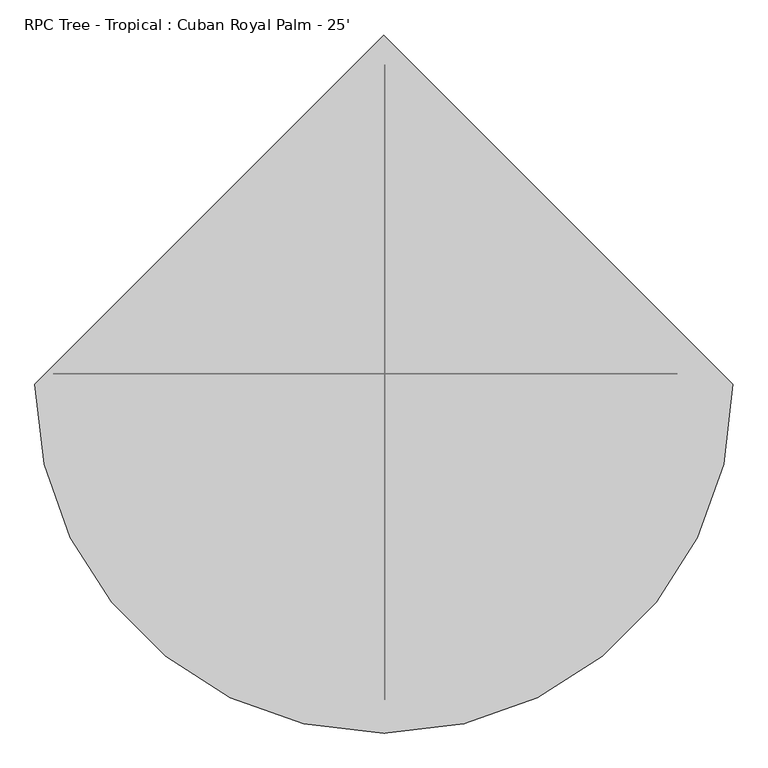
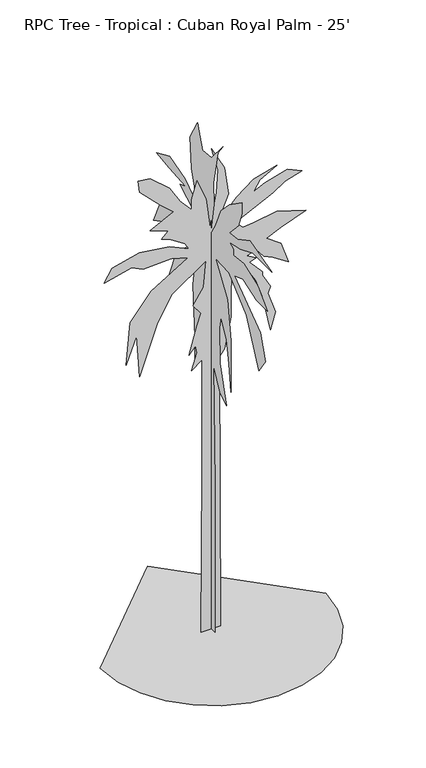
"""IFC4 building model written with IfcOpenShell, lengths in millimetres: geographic element geometry, RPC Tree - Tropical : Cuban Royal Palm - 25'."""

from ifc_helpers import new_model, si_unit, origin, place, context, project, spatial, triangles, source, transform, mapped, element, save


def rpc_tree_tropical_cuban_royal_palm_25_0a7aa95b(model_context):
    return source(origin(), model_context, "Body", "Tessellation", [
        triangles([(-108.765227, -0.0349819, 0.0018874), (-300.0839361, -0.0349989, 0.0018958), (-261.8198836, -0.0358763, 4989.2966217), (-261.8193749, -0.0364853, 8394.7422455), (-567.9281977, -0.0364309, 8165.1771881), (-414.8755486, -0.0365265, 8662.6107788), (-453.138075, -0.0365659, 8892.1752548), (-644.4583374, -0.0365165, 8662.6107788), (-414.8750399, -0.036677, 9504.4163727), (-300.0834274, -0.0367436, 9848.7895386), (-529.6656713, -0.0367883, 10154.9103882), (-223.556358, -0.0368838, 10614.0393402), (-147.0287708, -0.0370308, 11417.5937805), (-1141.8863325, -0.0368642, 10728.8474487), (-1562.7842606, -0.0367158, 10001.8499634), (-2098.4799053, -0.0364255, 8509.550354), (-2175.0048855, -0.0366548, 9810.5372223), (-2481.1151253, -0.0364977, 9006.9833633), (-2366.327655, -0.0367286, 10269.667337), (-1754.1070301, -0.0368921, 11034.9682983), (-682.7208275, -0.0370553, 11685.4611511), (-1180.1488953, -0.037061, 11838.5215759), (-1983.6872028, -0.037019, 11800.2181), (-2328.060078, -0.0370313, 11953.2785248), (-3131.5983856, -0.0369619, 11761.9657837), (-2902.0182129, -0.0370404, 12144.5912659), (-2098.4799053, -0.0371098, 12335.9551666), (-1218.4113853, -0.0371277, 12221.1470581), (-644.4583374, -0.0371049, 11953.2785248), (-759.2509672, -0.0371341, 12144.5912659), (-1218.4113853, -0.0371687, 12450.7121155), (-1447.996645, -0.0371724, 12527.2679077), (-1256.6789623, -0.037215, 12718.5806488), (-1792.3695202, -0.0372257, 12909.8922272), (-1103.6238424, -0.0373174, 13254.2653931), (-1486.2591351, -0.0373623, 13598.638559), (-2098.4799053, -0.037445, 14210.8790955), (-2136.7423954, -0.0375049, 14555.2522614), (-1792.3695202, -0.0375131, 14516.9487854), (-1218.4113853, -0.0374493, 14019.5163574), (-912.3010729, -0.0373737, 13522.0827667), (-567.9281977, -0.0373203, 13139.4572845), (-567.9281977, -0.037375, 13445.5781342), (-414.8750399, -0.0374776, 13981.2640411), (-147.0287708, -0.037373, 13330.7700256), (-32.2376989, -0.0372138, 12412.4597992), (159.0810602, -0.0374, 13407.3258179), (197.3450945, -0.0375249, 14096.0709869), (6.0263474, -0.0376465, 14823.069635), (388.6638127, -0.0375332, 14096.0709869), (503.4554252, -0.0373877, 13254.2653931), (159.0810602, -0.0372221, 12412.4597992), (733.0381777, -0.0373635, 13062.952652), (1230.4661728, -0.0374537, 13445.5781342), (1919.2119232, -0.037518, 13636.8908752), (1421.7838554, -0.0374483, 13369.0735016), (1230.4661728, -0.0373853, 13062.952652), (1574.839048, -0.0374277, 13216.0130768), (2225.3223083, -0.0374903, 13407.3258179), (2646.2251053, -0.0374745, 13216.0130768), (2148.7971828, -0.0374254, 13062.952652), (1804.4243076, -0.0373693, 12833.3375977), (694.7756876, -0.037225, 12297.6516907), (924.3558603, -0.037194, 12068.0866333), (1230.4661728, -0.0372142, 12106.3389496), (1919.2119232, -0.0372649, 12221.1470581), (2761.0178078, -0.0372537, 11953.2785248), (2034.0046257, -0.0371741, 11685.4611511), (1613.1015381, -0.0371215, 11494.14841), (2034.0046257, -0.0370851, 11188.0287231), (2263.5847984, -0.0369789, 10537.5347076), (1804.4243076, -0.0370135, 10843.6555573), (1536.5765579, -0.0370223, 10958.4125061), (1230.4661728, -0.0370774, 11341.0891479), (1230.4661728, -0.0370568, 11226.2810394), (1039.1484901, -0.0370348, 11149.7764069), (1306.9912983, -0.0370191, 10996.7159821), (1115.673543, -0.0369971, 10920.1601898), (1498.3140678, -0.0369385, 10499.2823914), (1498.3140678, -0.036918, 10384.4742828), (1727.8942406, -0.0368528, 9963.5976471), (1651.3692604, -0.0368152, 9772.284906), (1880.9494331, -0.036709, 9121.7914719), (1727.8942406, -0.0366133, 8624.3584625), (1498.3140678, -0.0368017, 9733.9814301), (1306.9912983, -0.036896, 10307.9696503), (962.6184231, -0.0369835, 10881.9078735), (618.2455479, -0.0369959, 11034.9682983), (579.9830215, -0.0368573, 10269.667337), (579.9830215, -0.0367068, 9427.9117401), (388.6638127, -0.0365343, 8509.550354), (235.6086383, -0.0364934, 8318.2376129), (273.8721821, -0.0350103, 0.0018707), (-0.007416, 179.1973287, 0.0009899), (-0.0074167, 327.2669789, 0.0010164), (-0.007416, 327.2669789, 3653.5578049), (-0.007412, 290.2500887, 8576.860199), (-0.0074152, 438.3187397, 8354.762709), (-0.0074113, 808.4913483, 7577.3712067), (-0.0074142, 808.4913483, 8502.8449493), (-0.0074136, 919.5451075, 10057.5767944), (-0.0074165, 771.4734043, 11131.0821991), (-0.0074182, 1067.6117237, 10797.8850952), (-0.0074135, 1585.8575615, 9724.3802719), (-0.0074128, 2178.1342003, 8984.0725525), (-0.0074169, 2622.3390633, 8280.7474594), (-0.0074142, 2104.0983124, 9687.3976456), (-0.0074148, 1770.942049, 10501.7717743), (-0.0074148, 1030.5937798, 11242.130072), (-0.007418, 1363.7500431, 11168.0636627), (-0.0074146, 1807.959993, 11131.0821991), (-0.0074152, 2215.1521442, 11205.0974487), (-0.0074151, 2918.4826149, 10834.9177185), (-0.0074174, 2548.3084076, 11649.2924286), (-0.0074135, 2141.1162563, 11649.2924286), (-0.0074142, 1993.0446259, 12278.6016907), (-0.0074152, 1289.7192421, 12130.5200317), (-0.0074177, 845.5092922, 12352.6169403), (-0.0074181, 1585.8575615, 12759.8292938), (-0.0074118, 1289.7192421, 12870.8783295), (-0.0074163, 2104.0983124, 12944.8935791), (-0.0074128, 2770.4108391, 13018.9599884), (-0.0074146, 2104.0983124, 13315.0733093), (-0.0074149, 1326.7371861, 13092.975238), (-0.0074185, 697.4375891, 12648.7814209), (-0.007414, 993.5809954, 13611.2366272), (-0.0074137, 1067.6117237, 14536.6592102), (-0.0074152, 697.4375891, 15202.9510986), (-0.0074137, 623.4067881, 14980.8541901), (-0.0074139, 438.3187397, 14499.6265869), (-0.0074172, -5.8891362, 14536.6592102), (-0.0074124, -598.1643245, 15239.9848846), (-0.0074156, -339.0454751, 14906.8389404), (-0.0074167, -116.9409725, 13833.3346985), (-0.0074169, -153.9583896, 13204.0242737), (-0.0074181, 31.1281259, 12167.552655), (-0.0074116, -227.9937325, 12574.7150116), (-0.0074171, -487.1146348, 13204.0242737), (-0.0074171, -931.3205515, 13648.2192535), (-0.007418, -1560.6150616, 14092.4642303), (-0.0074181, -1560.6150616, 13759.2682892), (-0.0074165, -1375.530574, 13278.090683), (-0.0074182, -931.3205515, 12796.8630798), (-0.0074127, -1338.5126301, 12833.8457062), (-0.0074184, -1967.8072128, 13166.9916504), (-0.0074149, -3078.3295441, 12870.8783295), (-0.0074161, -2115.8788433, 12870.8783295), (-0.0074144, -1486.5842606, 12611.7476349), (-0.0074166, -931.3205515, 12500.6985992), (-0.0074152, -1116.4101986, 12389.6507263), (-0.007416, -1116.4101986, 12204.586441), (-0.0074154, -1671.6688934, 12278.6016907), (-0.0074141, -2374.9992188, 12019.4709961), (-0.0074128, -2856.222171, 11538.2433929), (-0.0074175, -2300.9633308, 11538.2433929), (-0.0074131, -1597.6330055, 11760.3403015), (-0.0074162, -1190.4460138, 11612.3098022), (-0.0074138, -2486.0529053, 10649.8534332), (-0.0074142, -2745.1734261, 9909.4951355), (-0.0074134, -2412.0171627, 9428.2675323), (-0.0074143, -1782.72258, 10760.9024689), (-0.0074137, -894.3076944, 11538.2433929), (-0.0074119, -227.9937325, 11575.2760162), (-0.0074132, -820.2718792, 10649.8534332), (-0.0074137, -1005.3563667, 9502.282782), (-0.0074182, -1005.3563667, 7910.5683105), (-0.0074139, -894.3076944, 8724.9418579), (-0.007416, -783.2539352, 9391.2343277), (-0.0074166, -487.1146348, 9909.4951355), (-0.0074151, -413.0798006, 9539.3159866), (-0.007413, -450.0971995, 8465.8117447), (-0.0074184, -783.2539352, 7355.2737167), (-0.0074157, -450.0971995, 7577.3712067), (-0.007417, -116.9409725, 8206.6810501), (-0.0074127, -190.9763154, 4578.9905617), (-0.0074177, -190.9763154, 0.0009237), (-3306.1926704, -98.2582739, 0.0010848), (-3219.0250259, -853.7490509, 0.0009459), (-2970.7759346, -1547.5492893, 0.000811), (-2581.3232529, -2159.780088, 0.0006845), (-2070.5449825, -2670.5585037, 0.0005708), (-1458.3141838, -3060.0111855, 0.0004744), (-764.5188869, -3308.2602768, 0.0003997), (-9.0243572, -3395.4279213, 0.0003511), (746.469698, -3308.2602768, 0.0003337), (1440.2648495, -3060.0111855, 0.0003477), (2052.4957935, -2670.5585037, 0.0003906), (2563.2740639, -2159.780088, 0.0004596), (2952.7267456, -1547.5492893, 0.0005521), (3200.9758369, -853.7490509, 0.0006653), (3288.1434814, -98.2582739, 0.0007966), (-9.0249664, 3198.9082306, 0.0006054)], [[54, 55, 56], [48, 49, 50], [17, 18, 19], [15, 16, 17], [7, 8, 9], [83, 84, 85], [82, 83, 85], [4, 5, 6], [70, 71, 72], [66, 67, 68], [43, 44, 45], [59, 60, 61], [24, 25, 26], [24, 26, 27], [33, 34, 35], [76, 77, 78], [58, 59, 61], [58, 61, 62], [31, 32, 33], [42, 43, 45], [42, 45, 46], [37, 38, 39], [54, 56, 57], [53, 54, 57], [23, 24, 27], [23, 27, 28], [22, 23, 28], [22, 28, 29], [21, 22, 29], [58, 62, 63], [57, 58, 63], [53, 57, 63], [52, 53, 63], [36, 37, 39], [36, 39, 40], [36, 40, 41], [35, 36, 41], [35, 41, 42], [69, 70, 72], [69, 72, 73], [69, 73, 74], [65, 66, 68], [65, 68, 69], [65, 69, 74], [64, 65, 74], [47, 48, 50], [47, 50, 51], [46, 47, 51], [46, 51, 52], [33, 35, 42], [82, 85, 86], [81, 82, 86], [80, 81, 86], [33, 42, 46], [31, 33, 46], [30, 31, 46], [29, 30, 46], [15, 17, 19], [15, 19, 20], [14, 15, 20], [14, 20, 21], [13, 14, 21], [92, 93, 1], [92, 1, 2], [92, 2, 3], [92, 3, 4], [80, 86, 87], [79, 80, 87], [78, 79, 87], [76, 78, 87], [76, 87, 88], [13, 21, 29], [13, 29, 46], [13, 46, 52], [13, 52, 63], [13, 63, 64], [13, 64, 74], [13, 74, 75], [13, 75, 76], [13, 76, 88], [12, 13, 88], [12, 88, 89], [11, 12, 89], [10, 11, 89], [10, 89, 90], [9, 10, 90], [9, 90, 91], [7, 9, 91], [6, 7, 91], [4, 6, 91], [92, 4, 91], [131, 132, 133], [165, 166, 167], [105, 106, 107], [145, 146, 147], [165, 167, 168], [98, 99, 100], [131, 133, 134], [121, 122, 123], [104, 105, 107], [112, 113, 114], [171, 172, 173], [171, 173, 174], [153, 154, 155], [127, 128, 129], [118, 119, 120], [112, 114, 115], [139, 140, 141], [139, 141, 142], [159, 160, 161], [158, 159, 161], [157, 158, 161], [157, 161, 162], [104, 107, 108], [103, 104, 108], [103, 108, 109], [102, 103, 109], [127, 129, 130], [121, 123, 124], [120, 121, 124], [120, 124, 125], [118, 120, 125], [153, 155, 156], [152, 153, 156], [151, 152, 156], [151, 156, 157], [126, 127, 130], [145, 147, 148], [144, 145, 148], [144, 148, 149], [143, 144, 149], [139, 142, 143], [138, 139, 143], [137, 138, 143], [137, 143, 149], [175, 176, 94], [175, 94, 95], [175, 95, 96], [175, 96, 97], [174, 175, 97], [111, 112, 115], [115, 116, 117], [111, 115, 117], [110, 111, 117], [109, 110, 117], [165, 168, 169], [164, 165, 169], [130, 131, 134], [126, 130, 134], [126, 134, 135], [125, 126, 135], [125, 135, 136], [118, 125, 136], [151, 157, 162], [171, 174, 97], [170, 171, 97], [109, 117, 118], [109, 118, 136], [102, 109, 136], [97, 98, 100], [97, 100, 101], [170, 97, 101], [169, 170, 101], [169, 101, 102], [164, 169, 102], [163, 164, 102], [163, 102, 136], [151, 162, 163], [151, 163, 136], [151, 136, 137], [151, 137, 149], [151, 149, 150], [191, 192, 177], [190, 191, 177], [190, 177, 178], [189, 190, 178], [189, 178, 179], [189, 179, 180], [188, 189, 180], [187, 188, 180], [187, 180, 181], [187, 181, 182], [187, 182, 183], [187, 183, 184], [187, 184, 185], [187, 185, 186]], closed=False),
    ])


if __name__ == "__main__":
    model = new_model("IFC4")
    model_context = context("Model", 3, world=origin())
    ifc_project = project(units=[si_unit("LENGTHUNIT", "METRE", prefix="MILLI")], contexts=[model_context])
    site = spatial("IfcSite", under=ifc_project)
    building = spatial("IfcBuilding", under=site)
    placement = place(None, origin())
    rpc_tree_tropical_cuban_royal_palm_25_shape = rpc_tree_tropical_cuban_royal_palm_25_0a7aa95b(model_context)
    element("IfcGeographicElement", 1, ObjectType="RPC Tree - Tropical : Cuban Royal Palm - 25'", at=placement, inside=building, context=model_context, shape_type="MappedRepresentation", body=[
        mapped(rpc_tree_tropical_cuban_royal_palm_25_shape, transform((0.0, 0.0, 0.0), x_axis=(1.0, 0.0, 0.0), y_axis=(0.0, 1.0, 0.0), z_axis=(0.0, 0.0, 1.0))),
    ])
    save(model, "model.ifc")

# Revit data of these elements
# Type "RPC Tree - Tropical : Cuban Royal Palm - 25'"
#   built-in parameter 1005198 = "{2, 15},{39, RPC-16-FVGV-NKG0-7NHH-C000-ST1L-LVER-AU},{1, 0},{1, 0},{2, 13},{1, 8},{5, Color},{1, 0},{1, 0},{3, 0.8},{3, 0.8},{3, 0.8},{1, 8},{7, BBoxMin},{1, 0},{1, 0},{1, 0},{1, 0},{1, 0},{1, 8},{7, BBoxMax},{1, 0},{1, 0},{1, 0},{1, 0},{1, 0},{2, 11},{9, RPCTypeId},{1, 0},{1, 0},{39, RPC-16-FVGV-NKG0-7NHH-C000-ST1L-LVER-AU},{1, 6},{14, RPCPlantHeight},{1, 0},{1, 0},{2, 25},{2, 11},{7, keyword},{1, 0},{1, 0},{35, :RPCs:Trees [Tropical]:Geometry:RPC},{2, 11},{8, category},{1, 0},{1, 0},{16, Trees [Tropical]},{2, 11},{12, LocalizedUID},{1, 0},{1, 0},{16, Cuban Royal Palm},{2, 14},{6, Height},{1, 0},{1, 0},{2, 25},{1, 2},{16, Cast Reflections},{1, 0},{1, 0},{1, 0},{1, 2},{12, Cast Shadows},{1, 0},{1, 0},{1, 1},{1, 2},{9, Lock View},{1, 0},{1, 0},{1, 0},{1, 4},{5, ViewC},{1, 0},{1, 0},{1, 0},{21, assetlibrary_base.fbx},{1, 5},"
#   built-in parameter 1005195 = "RPC-16-FVGV-NKG0-7NHH-C000-ST1L-LVER-AU"
#   Type Comments = "Cuban Royal Palm"
#   Assembly Code = "G2050500"
#   Height = 50' - 0"
#   Plan Symbol = element 321958
#   Default Elevation = 0
